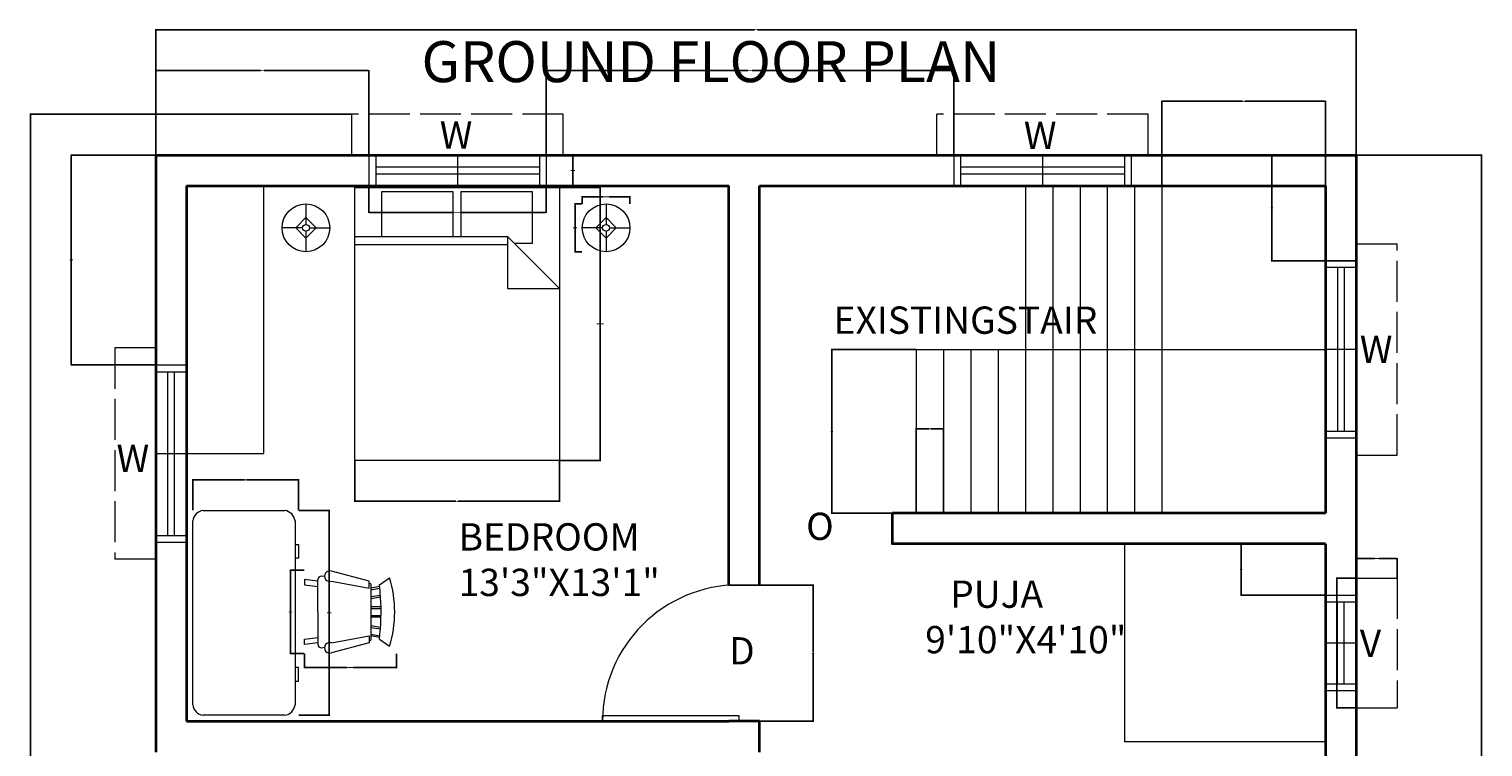
# Model space of a CAD drawing. Units: inches. Extents: x -35 to 832, y -515 to 219.
# Tile 5 of 7: x -35 to 391, y 9 to 219. Entities that reach past the tile are written whole.
import ezdxf

# ---------------------------------------------------------------- set-up
doc = ezdxf.new("R2010")
doc.units = ezdxf.units.IN
doc.header["$MEASUREMENT"] = 0
doc.linetypes.add('ACAD_ISO02W100', pattern=[15, 12, -3])
for name, color, linetype, lineweight in [('A-ANNO-TEXT', 7, 'Continuous', 18), ('A-AREA-IDEN', 7, 'Continuous', 18), ('A-DOOR', 4, 'Continuous', 18), ('A-FLOR-CASE', 3, 'Continuous', 18), ('A-FLOR-STRS', 2, 'Continuous', 18), ('A-FURN', 8, 'Continuous', 18), ('A-GLAZ', 2, 'Continuous', 18), ('A-GLAZ-OVHD', 2, 'ACAD_ISO02W100', 13), ('A-WALL', 10, 'Continuous', 35), ('G-ANNO-TEXT', 7, 'Continuous', 35), ('S-ANNO-DIMS', 2, 'Continuous', 18)]:
    doc.layers.add(name, color=color, linetype=linetype, lineweight=lineweight)
doc.styles.get("Standard").update_dxf_attribs({"font": 'arial.ttf'})
doc.dimstyles.get("Standard").update_dxf_attribs({"dimtxt": 0.18, "dimasz": 0.18, "dimexe": 0.18, "dimexo": 0.0625, "dimgap": 0.09, "dimtad": 0, "dimtih": 1, "dimtoh": 1, "dimdec": 1, "dimzin": 0, "dimdsep": 46, "dimlunit": 4, "dimtxsty": 'Standard', "dimcen": 0.09, "dimclrd": 211, "dimclre": 4, "dimclrt": 3, "dimadec": 0, "dimazin": 0, "dimtfac": 0.5, "dimtdec": 1, "dimtofl": 0, "dimtmove": 0, "dimatfit": 3, "dimfxl": 1, "dimtfill": 2, "dimtfillclr": 61, "dimtolj": 1, "dimtzin": 0, "dimarcsym": 0})

# ---------------------------------------------------------------- blocks, each defined once
blk = doc.blocks.new('*U5')
for p, q in [((0, 0), (0, -6)), ((40, 0), (40, -6))]:
    blk.add_line(p, q)
blk.add_lwpolyline([(0, 0), (0, 40), (1.75, 40), (1.75, 0)], close=True)
blk.add_arc((0, 0), 40, 0, 90)
blk = doc.blocks.new('Bed - Queen')
for p, q in [((0, -80.00003), (0, 0)), ((0, 0), (59.99999, 0)), ((59.99999, 0), (59.99999, -80.00003)), ((7.99999, -1.2), (28.79998, -1.2)), ((7.99999, -14.4), (7.99999, -1.2)), ((28.79998, -1.2), (28.79998, -14.4)), ((31.19999, -1.2), (51.99999, -1.2)), ((31.19999, -14.4), (31.19999, -1.2)), ((51.99999, -1.2), (51.99999, -16.4)), ((0, -14.4), (44.8, -14.4)), ((44.8, -16.8), (0, -16.8)), ((59.99999, -29.6), (44.8, -14.4)), ((44.8, -14.4), (44.8, -29.6)), ((51.99999, -16.4), (46.79936, -16.4)), ((44.8, -29.6), (59.99999, -29.6)), ((59.99999, -80.00003), (0, -80.00003))]:
    blk.add_line(p, q)
blk = doc.blocks.new('Chair - Rocking')
for p, q in [((-8, -4.5), (-10, -1.5)), ((-4.5, -7), (-4.96674, -4.19951)), ((-4, -7), (-4.40532, -4.16272)), ((-1.5, -4.05012), (-1.5, -7)), ((-1, -7), (-1, -4.05012)), ((1, -7), (1, -4.04655)), ((1.5, -4.05012), (1.5, -7)), ((4, -7), (4.40187, -4.18694)), ((4.5, -7), (4.96761, -4.19437)), ((8, -4.5), (10, -1.5)), ((-9, -7.5), (-12, -18.49999)), ((-7, -7.5), (-9, -7.5)), ((-9, -18.49999), (-7, -7.5)), ((-8.23428, -6.99939), (-8.3093, -7.47958)), ((-8.23041, -7), (8.23915, -7)), ((-7.5, -4.5), (-7, -7)), ((-6.5, -7), (-7.02225, -4.43)), ((6.5, -7), (7, -4.4057)), ((7.5, -4.5), (7, -7)), ((7, -7.5), (9, -7.5)), ((9, -18.49999), (7, -7.5)), ((8.31071, -7.48854), (8.23449, -7.00073)), ((9, -7.5), (12, -18.49999)), ((-10.36644, -20.64523), (-10.5, -21.49999)), ((10.5, -21.49999), (10.3575, -20.58798)), ((-9, -22.49999), (-9.5, -26.49999)), ((0, -22.49999), (-9.5, -22.49999)), ((-8, -26.49999), (-7.5, -22.49999)), ((0, -22.49999), (9.5, -22.49999)), ((8, -26.49999), (7.5, -22.49999)), ((9, -22.49999), (9.5, -26.49999)), ((-9.5, -26.49999), (-8, -26.49999)), ((9.5, -26.49999), (8, -26.49999))]:
    blk.add_line(p, q)
for centre, radius, start, end in [((0, -34.08333), 34.08333, 72.93847, 107.0615), ((0, -68.25004), 64.25, 93.92211, 97.15267), ((0, -68.25004), 64.25, 82.84733, 93.92211), ((-10.5, -18.99999), 1.58114, 161.5651, 18.43495), ((10.5, -18.99999), 1.58114, 161.5651, 18.43495), ((-9.5, -21.49999), 1, 180, 270), ((9.5, -21.49999), 1, 270, 0)]:
    blk.add_arc(centre, radius, start, end)
blk = doc.blocks.new('Desk - 30 x 60 in.')
for p, q in [((-26.999995, 0), (26.999995, 0)), ((-29.999995, -27), (-29.999995, -3)), ((29.999995, -3), (29.999995, -27)), ((26.999995, -30), (-26.999995, -30)), ((-20.000005, -30), (-20.000005, -31)), ((-20.000005, -31), (-16.000005, -31)), ((-16.000005, -31), (-16.000005, -30)), ((15.999995, -31), (15.999995, -30)), ((19.999995, -31), (15.999995, -31)), ((19.999995, -30), (19.999995, -31))]:
    blk.add_line(p, q)
for centre, start, end in [((-26.499995, -3.5), 98.1301, 171.8699), ((26.499995, -3.5), 8.130102, 81.8699), ((-26.499995, -26.5), 188.1301, 261.8699), ((26.499995, -26.5), 278.1301, 351.8699)]:
    blk.add_arc(centre, 3.535534, start, end)
blk = doc.blocks.new('Lamp - Table')
for p, q in [((0, 7), (0, 1)), ((-1, 0), (-7, 0)), ((0, 3), (-3, 0)), ((-3, 0), (0, -3)), ((3, 0), (0, 3)), ((0, -3), (3, 0)), ((1, 0), (7, 0)), ((0, -1), (0, -7))]:
    blk.add_line(p, q)
for radius in [7, 1]:
    blk.add_circle((0, 0), radius)
blk = doc.blocks.new('WIN-48')
for p, q in [((0, 9), (0, 0)), ((2, 9), (2, 0)), ((26, 9), (26, 0)), ((50, 9), (50, 0)), ((52, 9), (52, 0)), ((2, 5.5), (50, 5.5)), ((2, 3.5), (50, 3.5))]:
    blk.add_line(p, q)
blk = doc.blocks.new('VENT-24')
for p, q in [((9, 28), (0, 28)), ((9, 26), (0, 26)), ((3.5, 26), (3.5, 2)), ((5.5, 26), (5.5, 2)), ((9, 14), (0, 14)), ((9, 2), (0, 2)), ((9, 0), (0, 0))]:
    blk.add_line(p, q)
blk = doc.blocks.new('WIN-48-HOOD')
for p, q in [((5, 12), (0, 12)), ((0, 12), (0, 0)), ((57, 12), (62, 12)), ((62, 12), (62, 0)), ((0, 0), (62, 0))]:
    blk.add_line(p, q)
blk = doc.blocks.new('VENT-24-HOOD')
for p, q in [((12, 38), (0, 38)), ((0, 0), (0, 38)), ((12, 33), (12, 38)), ((12, 5), (12, 0)), ((12, 0), (0, 0))]:
    blk.add_line(p, q)
blk = doc.blocks.new('*D61')
at = {"layer": 'Defpoints', "color": 0, "transparency": 16777216}
for p in [(64.3, 173.05), (116.3, 173.05), (116.3, 165.25)]:
    blk.add_point(p, dxfattribs=at)
at = {"layer": 'S-ANNO-DIMS', "color": 4, "lineweight": -2, "transparency": 16777216}
for p, q in [((64.3, 172.99), (64.3, 165.07)), ((116.3, 172.99), (116.3, 165.07))]:
    blk.add_line(p, q, dxfattribs=at)
at = {"layer": 'S-ANNO-DIMS', "color": 211, "lineweight": -2, "transparency": 16777216}
for p, q in [((64.48, 165.25), (89.07, 165.25)), ((116.12, 165.25), (91.53, 165.25))]:
    blk.add_line(p, q, dxfattribs=at)
at = {"layer": 'S-ANNO-DIMS', "color": 211, "transparency": 16777216}
for points in [[(64.48, 165.28), (64.48, 165.22), (64.3, 165.25)], [(116.12, 165.28), (116.12, 165.22), (116.3, 165.25)]]:
    blk.add_solid(points, dxfattribs=at)
at = {"layer": 'S-ANNO-DIMS', "color": 3, "transparency": 16777216, "insert": (90.3, 165.25), "char_height": 0.18, "attachment_point": 5, "bg_fill": 1, "box_fill_scale": 1.25, "bg_fill_color": 61, "bg_fill_transparency": 0}
blk.add_mtext('\\A1;WINDOW 4\'-4" TYP.', dxfattribs=at)
blk = doc.blocks.new('*D62')
at = {"layer": 'Defpoints', "color": 0, "transparency": 16777216}
for p in [(116.3, 182.05), (124.1, 182.05), (116.3, 173.05)]:
    blk.add_point(p, dxfattribs=at)
at = {"layer": 'S-ANNO-DIMS', "color": 4, "lineweight": -2, "transparency": 16777216}
for p, q in [((116.36, 182.05), (124.28, 182.05)), ((116.36, 173.05), (124.28, 173.05))]:
    blk.add_line(p, q, dxfattribs=at)
at = {"layer": 'S-ANNO-DIMS', "color": 211, "lineweight": -2, "transparency": 16777216}
for p, q in [((124.1, 181.87), (124.1, 177.73)), ((124.1, 173.23), (124.1, 177.37))]:
    blk.add_line(p, q, dxfattribs=at)
at = {"layer": 'S-ANNO-DIMS', "color": 211, "transparency": 16777216}
for points in [[(124.07, 181.87), (124.13, 181.87), (124.1, 182.05)], [(124.07, 173.23), (124.13, 173.23), (124.1, 173.05)]]:
    blk.add_solid(points, dxfattribs=at)
at = {"layer": 'S-ANNO-DIMS', "color": 3, "transparency": 16777216, "insert": (124.1, 177.55), "char_height": 0.18, "attachment_point": 5, "bg_fill": 1, "box_fill_scale": 1.25, "bg_fill_color": 61, "bg_fill_transparency": 0}
blk.add_mtext('\\A1;0\'-9" TYP.', dxfattribs=at)
blk = doc.blocks.new('*D67')
at = {"layer": 'Defpoints', "color": 0, "transparency": 16777216}
for p in [(353.8, 58.05), (348.1, 20.05), (353.8, 20.05)]:
    blk.add_point(p, dxfattribs=at)
at = {"layer": 'S-ANNO-DIMS', "color": 4, "lineweight": -2, "transparency": 16777216}
for p, q in [((353.74, 58.05), (347.92, 58.05)), ((353.74, 20.05), (347.92, 20.05))]:
    blk.add_line(p, q, dxfattribs=at)
at = {"layer": 'S-ANNO-DIMS', "color": 211, "lineweight": -2, "transparency": 16777216}
for p, q in [((348.1, 57.87), (348.1, 39.23)), ((348.1, 20.23), (348.1, 38.87))]:
    blk.add_line(p, q, dxfattribs=at)
at = {"layer": 'S-ANNO-DIMS', "color": 211, "transparency": 16777216}
for points in [[(348.07, 57.87), (348.13, 57.87), (348.1, 58.05)], [(348.07, 20.23), (348.13, 20.23), (348.1, 20.05)]]:
    blk.add_solid(points, dxfattribs=at)
at = {"layer": 'S-ANNO-DIMS', "color": 3, "transparency": 16777216, "insert": (348.1, 39.05), "char_height": 0.18, "attachment_point": 5, "bg_fill": 1, "box_fill_scale": 1.25, "bg_fill_color": 61, "bg_fill_transparency": 0}
blk.add_mtext('\\A1;VENT HOOD 3\'-2" TYP.', dxfattribs=at)
blk = doc.blocks.new('*D68')
at = {"layer": 'Defpoints', "color": 0, "transparency": 16777216}
for p in [(353.8, 63.75), (353.8, 58.05), (365.8, 58.05)]:
    blk.add_point(p, dxfattribs=at)
at = {"layer": 'S-ANNO-DIMS', "color": 4, "lineweight": -2, "transparency": 16777216}
for p, q in [((353.8, 58.11), (353.8, 63.93)), ((365.8, 58.11), (365.8, 63.93))]:
    blk.add_line(p, q, dxfattribs=at)
at = {"layer": 'S-ANNO-DIMS', "color": 211, "lineweight": -2, "transparency": 16777216}
for p, q in [((353.98, 63.75), (359.17, 63.75)), ((365.62, 63.75), (360.43, 63.75))]:
    blk.add_line(p, q, dxfattribs=at)
at = {"layer": 'S-ANNO-DIMS', "color": 211, "transparency": 16777216}
for points in [[(353.98, 63.78), (353.98, 63.72), (353.8, 63.75)], [(365.62, 63.78), (365.62, 63.72), (365.8, 63.75)]]:
    blk.add_solid(points, dxfattribs=at)
at = {"layer": 'S-ANNO-DIMS', "color": 3, "transparency": 16777216, "insert": (359.8, 63.75), "char_height": 0.18, "attachment_point": 5, "bg_fill": 1, "box_fill_scale": 1.25, "bg_fill_color": 61, "bg_fill_transparency": 0}
blk.add_mtext('\\A1;1\'-0" TYP.', dxfattribs=at)
blk = doc.blocks.new('*D73')
at = {"layer": 'Defpoints', "color": 0, "transparency": 16777216}
for p in [(126.84, 167.72), (140.84, 169.82), (140.84, 167.72)]:
    blk.add_point(p, dxfattribs=at)
at = {"layer": 'S-ANNO-DIMS', "color": 4, "lineweight": -2, "transparency": 16777216}
for p, q in [((126.84, 167.79), (126.84, 170)), ((140.84, 167.79), (140.84, 170))]:
    blk.add_line(p, q, dxfattribs=at)
at = {"layer": 'S-ANNO-DIMS', "color": 211, "lineweight": -2, "transparency": 16777216}
for p, q in [((127.02, 169.82), (132.83, 169.82)), ((140.66, 169.82), (134.85, 169.82))]:
    blk.add_line(p, q, dxfattribs=at)
at = {"layer": 'S-ANNO-DIMS', "color": 211, "transparency": 16777216}
for points in [[(127.02, 169.85), (127.02, 169.79), (126.84, 169.82)], [(140.66, 169.85), (140.66, 169.79), (140.84, 169.82)]]:
    blk.add_solid(points, dxfattribs=at)
at = {"layer": 'S-ANNO-DIMS', "color": 3, "transparency": 16777216, "insert": (133.84, 169.82), "char_height": 0.18, "attachment_point": 5, "bg_fill": 1, "box_fill_scale": 1.25, "bg_fill_color": 61, "bg_fill_transparency": 0}
blk.add_mtext('\\A1;LAMP 1\'-2" TYP.', dxfattribs=at)
blk = doc.blocks.new('*D74')
at = {"layer": 'Defpoints', "color": 0, "transparency": 16777216}
for p in [(124.74, 167.72), (126.84, 167.72), (126.84, 153.72)]:
    blk.add_point(p, dxfattribs=at)
at = {"layer": 'S-ANNO-DIMS', "color": 4, "lineweight": -2, "transparency": 16777216}
for p, q in [((126.78, 167.72), (124.56, 167.72)), ((126.78, 153.72), (124.56, 153.72))]:
    blk.add_line(p, q, dxfattribs=at)
at = {"layer": 'S-ANNO-DIMS', "color": 211, "lineweight": -2, "transparency": 16777216}
for p, q in [((124.74, 167.54), (124.74, 160.9)), ((124.74, 153.9), (124.74, 160.54))]:
    blk.add_line(p, q, dxfattribs=at)
at = {"layer": 'S-ANNO-DIMS', "color": 211, "transparency": 16777216}
for points in [[(124.71, 167.54), (124.77, 167.54), (124.74, 167.72)], [(124.71, 153.9), (124.77, 153.9), (124.74, 153.72)]]:
    blk.add_solid(points, dxfattribs=at)
at = {"layer": 'S-ANNO-DIMS', "color": 3, "transparency": 16777216, "insert": (124.74, 160.72), "char_height": 0.18, "attachment_point": 5, "bg_fill": 1, "box_fill_scale": 1.25, "bg_fill_color": 61, "bg_fill_transparency": 0}
blk.add_mtext('\\A1;1\'-2" TYP.', dxfattribs=at)
blk = doc.blocks.new('*D89')
at = {"layer": 'Defpoints', "color": 0, "transparency": 16777216}
for p in [(120.14, 172.55), (132.14, 172.55), (120.14, 92.55)]:
    blk.add_point(p, dxfattribs=at)
at = {"layer": 'S-ANNO-DIMS', "color": 4, "lineweight": -2, "transparency": 16777216}
for p, q in [((120.2, 172.55), (132.32, 172.55)), ((120.2, 92.55), (132.32, 92.55))]:
    blk.add_line(p, q, dxfattribs=at)
at = {"layer": 'S-ANNO-DIMS', "color": 211, "lineweight": -2, "transparency": 16777216}
for p, q in [((132.14, 172.37), (132.14, 132.74)), ((132.14, 92.73), (132.14, 132.36))]:
    blk.add_line(p, q, dxfattribs=at)
at = {"layer": 'S-ANNO-DIMS', "color": 211, "transparency": 16777216}
for points in [[(132.11, 172.37), (132.17, 172.37), (132.14, 172.55)], [(132.11, 92.73), (132.17, 92.73), (132.14, 92.55)]]:
    blk.add_solid(points, dxfattribs=at)
at = {"layer": 'S-ANNO-DIMS', "color": 3, "transparency": 16777216, "insert": (132.14, 132.55), "char_height": 0.18, "attachment_point": 5, "bg_fill": 1, "box_fill_scale": 1.25, "bg_fill_color": 61, "bg_fill_transparency": 0}
blk.add_mtext('\\A1;QUEEN BED 6\'-8"', dxfattribs=at)
blk = doc.blocks.new('*D90')
at = {"layer": 'Defpoints', "color": 0, "transparency": 16777216}
for p in [(60.14, 92.55), (120.14, 92.55), (120.14, 80.55)]:
    blk.add_point(p, dxfattribs=at)
at = {"layer": 'S-ANNO-DIMS', "color": 4, "lineweight": -2, "transparency": 16777216}
for p, q in [((60.14, 92.49), (60.14, 80.37)), ((120.14, 92.49), (120.14, 80.37))]:
    blk.add_line(p, q, dxfattribs=at)
at = {"layer": 'S-ANNO-DIMS', "color": 211, "lineweight": -2, "transparency": 16777216}
for p, q in [((60.32, 80.55), (89.81, 80.55)), ((119.96, 80.55), (90.47, 80.55))]:
    blk.add_line(p, q, dxfattribs=at)
at = {"layer": 'S-ANNO-DIMS', "color": 211, "transparency": 16777216}
for points in [[(60.32, 80.58), (60.32, 80.52), (60.14, 80.55)], [(119.96, 80.58), (119.96, 80.52), (120.14, 80.55)]]:
    blk.add_solid(points, dxfattribs=at)
at = {"layer": 'S-ANNO-DIMS', "color": 3, "transparency": 16777216, "insert": (90.14, 80.55), "char_height": 0.18, "attachment_point": 5, "bg_fill": 1, "box_fill_scale": 1.25, "bg_fill_color": 61, "bg_fill_transparency": 0}
blk.add_mtext('\\A1;5\'-0"', dxfattribs=at)
blk = doc.blocks.new('*D91')
at = {"layer": 'Defpoints', "color": 0, "transparency": 16777216}
for p in [(45.37, 35.89), (72.37, 35.89), (72.37, 31.84)]:
    blk.add_point(p, dxfattribs=at)
at = {"layer": 'S-ANNO-DIMS', "color": 4, "lineweight": -2, "transparency": 16777216}
for p, q in [((45.37, 35.82), (45.37, 31.66)), ((72.37, 35.82), (72.37, 31.66))]:
    blk.add_line(p, q, dxfattribs=at)
at = {"layer": 'S-ANNO-DIMS', "color": 211, "lineweight": -2, "transparency": 16777216}
for p, q in [((45.55, 31.84), (57.97, 31.84)), ((72.19, 31.84), (59.77, 31.84))]:
    blk.add_line(p, q, dxfattribs=at)
at = {"layer": 'S-ANNO-DIMS', "color": 211, "transparency": 16777216}
for points in [[(45.55, 31.87), (45.55, 31.81), (45.37, 31.84)], [(72.19, 31.87), (72.19, 31.81), (72.37, 31.84)]]:
    blk.add_solid(points, dxfattribs=at)
at = {"layer": 'S-ANNO-DIMS', "color": 3, "transparency": 16777216, "insert": (58.87, 31.84), "char_height": 0.18, "attachment_point": 5, "bg_fill": 1, "box_fill_scale": 1.25, "bg_fill_color": 61, "bg_fill_transparency": 0}
blk.add_mtext('\\A1;ROCKER 2\'-3"', dxfattribs=at)
blk = doc.blocks.new('*D92')
at = {"layer": 'Defpoints', "color": 0, "transparency": 16777216}
for p in [(45.37, 60.32), (41.32, 35.89), (45.37, 35.89)]:
    blk.add_point(p, dxfattribs=at)
at = {"layer": 'S-ANNO-DIMS', "color": 4, "lineweight": -2, "transparency": 16777216}
for p, q in [((45.31, 60.32), (41.14, 60.32)), ((45.31, 35.89), (41.14, 35.89))]:
    blk.add_line(p, q, dxfattribs=at)
at = {"layer": 'S-ANNO-DIMS', "color": 211, "lineweight": -2, "transparency": 16777216}
for p, q in [((41.32, 60.14), (41.32, 48.29)), ((41.32, 36.07), (41.32, 47.92))]:
    blk.add_line(p, q, dxfattribs=at)
at = {"layer": 'S-ANNO-DIMS', "color": 211, "transparency": 16777216}
for points in [[(41.29, 60.14), (41.35, 60.14), (41.32, 60.32)], [(41.29, 36.07), (41.35, 36.07), (41.32, 35.89)]]:
    blk.add_solid(points, dxfattribs=at)
at = {"layer": 'S-ANNO-DIMS', "color": 3, "transparency": 16777216, "insert": (41.32, 48.1), "char_height": 0.18, "attachment_point": 5, "bg_fill": 1, "box_fill_scale": 1.25, "bg_fill_color": 61, "bg_fill_transparency": 0}
blk.add_mtext('\\A1;2\'-0 1/2"', dxfattribs=at)
blk = doc.blocks.new('*D93')
at = {"layer": 'Defpoints', "color": 0, "transparency": 16777216}
for p in [(43.66, 77.85), (52.66, 77.85), (43.66, 17.85)]:
    blk.add_point(p, dxfattribs=at)
at = {"layer": 'S-ANNO-DIMS', "color": 4, "lineweight": -2, "transparency": 16777216}
for p, q in [((43.72, 77.85), (52.84, 77.85)), ((43.72, 17.85), (52.84, 17.85))]:
    blk.add_line(p, q, dxfattribs=at)
at = {"layer": 'S-ANNO-DIMS', "color": 211, "lineweight": -2, "transparency": 16777216}
for p, q in [((52.66, 77.67), (52.66, 48.03)), ((52.66, 18.03), (52.66, 47.67))]:
    blk.add_line(p, q, dxfattribs=at)
at = {"layer": 'S-ANNO-DIMS', "color": 211, "transparency": 16777216}
for points in [[(52.63, 77.67), (52.69, 77.67), (52.66, 77.85)], [(52.63, 18.03), (52.69, 18.03), (52.66, 17.85)]]:
    blk.add_solid(points, dxfattribs=at)
at = {"layer": 'S-ANNO-DIMS', "color": 3, "transparency": 16777216, "insert": (52.66, 47.85), "char_height": 0.18, "attachment_point": 5, "bg_fill": 1, "box_fill_scale": 1.25, "bg_fill_color": 61, "bg_fill_transparency": 0}
blk.add_mtext('\\A1;DESK 5\'-0"', dxfattribs=at)
blk = doc.blocks.new('*D94')
at = {"layer": 'Defpoints', "color": 0, "transparency": 16777216}
for p in [(12.66, 86.85), (12.66, 77.85), (43.66, 77.85)]:
    blk.add_point(p, dxfattribs=at)
at = {"layer": 'S-ANNO-DIMS', "color": 4, "lineweight": -2, "transparency": 16777216}
for p, q in [((12.66, 77.91), (12.66, 87.03)), ((43.66, 77.91), (43.66, 87.03))]:
    blk.add_line(p, q, dxfattribs=at)
at = {"layer": 'S-ANNO-DIMS', "color": 211, "lineweight": -2, "transparency": 16777216}
for p, q in [((12.84, 86.85), (27.83, 86.85)), ((43.48, 86.85), (28.49, 86.85))]:
    blk.add_line(p, q, dxfattribs=at)
at = {"layer": 'S-ANNO-DIMS', "color": 211, "transparency": 16777216}
for points in [[(12.84, 86.88), (12.84, 86.82), (12.66, 86.85)], [(43.48, 86.88), (43.48, 86.82), (43.66, 86.85)]]:
    blk.add_solid(points, dxfattribs=at)
at = {"layer": 'S-ANNO-DIMS', "color": 3, "transparency": 16777216, "insert": (28.16, 86.85), "char_height": 0.18, "attachment_point": 5, "bg_fill": 1, "box_fill_scale": 1.25, "bg_fill_color": 61, "bg_fill_transparency": 0}
blk.add_mtext('\\A1;2\'-7"', dxfattribs=at)
blk = doc.blocks.new('*D103')
at = {"layer": 'Defpoints', "color": 0, "transparency": 16777216}
for p in [(64.3, 206.8), (1.8, 182.05), (64.3, 182.05)]:
    blk.add_point(p, dxfattribs=at)
at = {"layer": 'S-ANNO-DIMS', "color": 4, "lineweight": -2, "transparency": 16777216}
for p, q in [((1.8, 182.11), (1.8, 206.98)), ((64.3, 182.11), (64.3, 206.98))]:
    blk.add_line(p, q, dxfattribs=at)
at = {"layer": 'S-ANNO-DIMS', "color": 211, "lineweight": -2, "transparency": 16777216}
for p, q in [((1.98, 206.8), (32.51, 206.8)), ((64.12, 206.8), (33.59, 206.8))]:
    blk.add_line(p, q, dxfattribs=at)
at = {"layer": 'S-ANNO-DIMS', "color": 211, "transparency": 16777216}
for points in [[(1.98, 206.83), (1.98, 206.77), (1.8, 206.8)], [(64.12, 206.83), (64.12, 206.77), (64.3, 206.8)]]:
    blk.add_solid(points, dxfattribs=at)
at = {"layer": 'S-ANNO-DIMS', "color": 3, "transparency": 16777216, "insert": (33.05, 206.8), "char_height": 0.18, "attachment_point": 5, "bg_fill": 1, "box_fill_scale": 1.25, "bg_fill_color": 61, "bg_fill_transparency": 0}
blk.add_mtext('\\A1;5\'-2 1/2"', dxfattribs=at)
blk = doc.blocks.new('*D104')
at = {"layer": 'Defpoints', "color": 0, "transparency": 16777216}
for p in [(235.8, 206.8), (116.3, 182.05), (235.8, 182.05)]:
    blk.add_point(p, dxfattribs=at)
at = {"layer": 'S-ANNO-DIMS', "color": 4, "lineweight": -2, "transparency": 16777216}
for p, q in [((116.3, 182.11), (116.3, 206.98)), ((235.8, 182.11), (235.8, 206.98))]:
    blk.add_line(p, q, dxfattribs=at)
at = {"layer": 'S-ANNO-DIMS', "color": 211, "lineweight": -2, "transparency": 16777216}
for p, q in [((116.48, 206.8), (175.44, 206.8)), ((235.62, 206.8), (176.66, 206.8))]:
    blk.add_line(p, q, dxfattribs=at)
at = {"layer": 'S-ANNO-DIMS', "color": 211, "transparency": 16777216}
for points in [[(116.48, 206.83), (116.48, 206.77), (116.3, 206.8)], [(235.62, 206.83), (235.62, 206.77), (235.8, 206.8)]]:
    blk.add_solid(points, dxfattribs=at)
at = {"layer": 'S-ANNO-DIMS', "color": 3, "transparency": 16777216, "insert": (176.05, 206.8), "char_height": 0.18, "attachment_point": 5, "bg_fill": 1, "box_fill_scale": 1.25, "bg_fill_color": 61, "bg_fill_transparency": 0}
blk.add_mtext('\\A1;9\'-11 1/2"', dxfattribs=at)
blk = doc.blocks.new('*D105')
at = {"layer": 'Defpoints', "color": 0, "transparency": 16777216}
for p in [(353.8, 218.8), (1.8, 182.05), (353.8, 182.05)]:
    blk.add_point(p, dxfattribs=at)
at = {"layer": 'S-ANNO-DIMS', "color": 4, "lineweight": -2, "transparency": 16777216}
for p, q in [((1.8, 182.11), (1.8, 218.98)), ((353.8, 182.11), (353.8, 218.98))]:
    blk.add_line(p, q, dxfattribs=at)
at = {"layer": 'S-ANNO-DIMS', "color": 211, "lineweight": -2, "transparency": 16777216}
for p, q in [((1.98, 218.8), (177.4, 218.8)), ((353.62, 218.8), (178.2, 218.8))]:
    blk.add_line(p, q, dxfattribs=at)
at = {"layer": 'S-ANNO-DIMS', "color": 211, "transparency": 16777216}
for points in [[(1.98, 218.83), (1.98, 218.77), (1.8, 218.8)], [(353.62, 218.83), (353.62, 218.77), (353.8, 218.8)]]:
    blk.add_solid(points, dxfattribs=at)
at = {"layer": 'S-ANNO-DIMS', "color": 3, "transparency": 16777216, "insert": (177.8, 218.8), "char_height": 0.18, "attachment_point": 5, "bg_fill": 1, "box_fill_scale": 1.25, "bg_fill_color": 61, "bg_fill_transparency": 0}
blk.add_mtext('\\A1;29\'-4"', dxfattribs=at)
blk = doc.blocks.new('*D106')
at = {"layer": 'Defpoints', "color": 0, "transparency": 16777216}
for p in [(353.8, 182.05), (353.8, -254.95), (390.55, -254.95)]:
    blk.add_point(p, dxfattribs=at)
at = {"layer": 'S-ANNO-DIMS', "color": 4, "lineweight": -2, "transparency": 16777216}
for p, q in [((353.86, 182.05), (390.73, 182.05)), ((353.86, -254.95), (390.73, -254.95))]:
    blk.add_line(p, q, dxfattribs=at)
at = {"layer": 'S-ANNO-DIMS', "color": 211, "lineweight": -2, "transparency": 16777216}
for p, q in [((390.55, 181.87), (390.55, -36.27)), ((390.55, -254.77), (390.55, -36.63))]:
    blk.add_line(p, q, dxfattribs=at)
at = {"layer": 'S-ANNO-DIMS', "color": 211, "transparency": 16777216}
for points in [[(390.52, 181.87), (390.58, 181.87), (390.55, 182.05)], [(390.52, -254.77), (390.58, -254.77), (390.55, -254.95)]]:
    blk.add_solid(points, dxfattribs=at)
at = {"layer": 'S-ANNO-DIMS', "color": 3, "transparency": 16777216, "insert": (390.55, -36.45), "char_height": 0.18, "attachment_point": 5, "bg_fill": 1, "box_fill_scale": 1.25, "bg_fill_color": 61, "bg_fill_transparency": 0}
blk.add_mtext('\\A1;36\'-5"', dxfattribs=at)
blk = doc.blocks.new('*D110')
at = {"layer": 'Defpoints', "color": 0, "transparency": 16777216}
for p in [(59.3, 194.05), (-34.95, -254.95), (129.8, -254.95)]:
    blk.add_point(p, dxfattribs=at)
at = {"layer": 'S-ANNO-DIMS', "color": 4, "lineweight": -2, "transparency": 16777216}
for p, q in [((59.24, 194.05), (-35.13, 194.05)), ((129.74, -254.95), (-35.13, -254.95))]:
    blk.add_line(p, q, dxfattribs=at)
at = {"layer": 'S-ANNO-DIMS', "color": 211, "lineweight": -2, "transparency": 16777216}
for p, q in [((-34.95, 193.87), (-34.95, -30.27)), ((-34.95, -254.77), (-34.95, -30.63))]:
    blk.add_line(p, q, dxfattribs=at)
at = {"layer": 'S-ANNO-DIMS', "color": 211, "transparency": 16777216}
for points in [[(-34.98, 193.87), (-34.92, 193.87), (-34.95, 194.05)], [(-34.98, -254.77), (-34.92, -254.77), (-34.95, -254.95)]]:
    blk.add_solid(points, dxfattribs=at)
at = {"layer": 'S-ANNO-DIMS', "color": 3, "transparency": 16777216, "insert": (-34.95, -30.45), "char_height": 0.18, "attachment_point": 5, "bg_fill": 1, "box_fill_scale": 1.25, "bg_fill_color": 61, "bg_fill_transparency": 0}
blk.add_mtext('\\A1;37\'-5"', dxfattribs=at)
blk = doc.blocks.new('*D112')
at = {"layer": 'Defpoints', "color": 0, "transparency": 16777216}
for p in [(169.8, 55.94), (169.8, 16.05), (194.55, 16.05)]:
    blk.add_point(p, dxfattribs=at)
at = {"layer": 'S-ANNO-DIMS', "color": 4, "lineweight": -2, "transparency": 16777216}
for p, q in [((169.86, 55.94), (194.73, 55.94)), ((169.86, 16.05), (194.73, 16.05))]:
    blk.add_line(p, q, dxfattribs=at)
at = {"layer": 'S-ANNO-DIMS', "color": 211, "lineweight": -2, "transparency": 16777216}
for p, q in [((194.55, 55.76), (194.55, 36.18)), ((194.55, 16.23), (194.55, 35.81))]:
    blk.add_line(p, q, dxfattribs=at)
at = {"layer": 'S-ANNO-DIMS', "color": 211, "transparency": 16777216}
for points in [[(194.52, 55.76), (194.58, 55.76), (194.55, 55.94)], [(194.52, 16.23), (194.58, 16.23), (194.55, 16.05)]]:
    blk.add_solid(points, dxfattribs=at)
at = {"layer": 'S-ANNO-DIMS', "color": 3, "transparency": 16777216, "insert": (194.55, 35.99), "char_height": 0.18, "attachment_point": 5, "bg_fill": 1, "box_fill_scale": 1.25, "bg_fill_color": 61, "bg_fill_transparency": 0}
blk.add_mtext('\\A1;3\'-4"', dxfattribs=at)
blk = doc.blocks.new('*D115')
at = {"layer": 'Defpoints', "color": 0, "transparency": 16777216}
for p in [(-22.95, 182.05), (1.8, 182.05), (1.8, 120.55)]:
    blk.add_point(p, dxfattribs=at)
at = {"layer": 'S-ANNO-DIMS', "color": 4, "lineweight": -2, "transparency": 16777216}
for p, q in [((1.74, 182.05), (-23.13, 182.05)), ((1.74, 120.55), (-23.13, 120.55))]:
    blk.add_line(p, q, dxfattribs=at)
at = {"layer": 'S-ANNO-DIMS', "color": 211, "lineweight": -2, "transparency": 16777216}
for p, q in [((-22.95, 181.87), (-22.95, 151.48)), ((-22.95, 120.73), (-22.95, 151.12))]:
    blk.add_line(p, q, dxfattribs=at)
at = {"layer": 'S-ANNO-DIMS', "color": 211, "transparency": 16777216}
for points in [[(-22.98, 181.87), (-22.92, 181.87), (-22.95, 182.05)], [(-22.98, 120.73), (-22.92, 120.73), (-22.95, 120.55)]]:
    blk.add_solid(points, dxfattribs=at)
at = {"layer": 'S-ANNO-DIMS', "color": 3, "transparency": 16777216, "insert": (-22.95, 151.3), "char_height": 0.18, "attachment_point": 5, "bg_fill": 1, "box_fill_scale": 1.25, "bg_fill_color": 61, "bg_fill_transparency": 0}
blk.add_mtext('\\A1;5\'-1 1/2"', dxfattribs=at)
blk = doc.blocks.new('*D118')
at = {"layer": 'Defpoints', "color": 0, "transparency": 16777216}
for p in [(329.05, 182.05), (353.8, 182.05), (353.8, 151.05)]:
    blk.add_point(p, dxfattribs=at)
at = {"layer": 'S-ANNO-DIMS', "color": 4, "lineweight": -2, "transparency": 16777216}
for p, q in [((353.74, 182.05), (328.87, 182.05)), ((353.74, 151.05), (328.87, 151.05))]:
    blk.add_line(p, q, dxfattribs=at)
at = {"layer": 'S-ANNO-DIMS', "color": 211, "lineweight": -2, "transparency": 16777216}
for p, q in [((329.05, 181.87), (329.05, 166.73)), ((329.05, 151.23), (329.05, 166.37))]:
    blk.add_line(p, q, dxfattribs=at)
at = {"layer": 'S-ANNO-DIMS', "color": 211, "transparency": 16777216}
for points in [[(329.02, 181.87), (329.08, 181.87), (329.05, 182.05)], [(329.02, 151.23), (329.08, 151.23), (329.05, 151.05)]]:
    blk.add_solid(points, dxfattribs=at)
at = {"layer": 'S-ANNO-DIMS', "color": 3, "transparency": 16777216, "insert": (329.05, 166.55), "char_height": 0.18, "attachment_point": 5, "bg_fill": 1, "box_fill_scale": 1.25, "bg_fill_color": 61, "bg_fill_transparency": 0}
blk.add_mtext('\\A1;2\'-7"', dxfattribs=at)
blk = doc.blocks.new('*D119')
at = {"layer": 'Defpoints', "color": 0, "transparency": 16777216}
for p in [(320.05, 68.05), (344.8, 68.05), (344.8, 53.05)]:
    blk.add_point(p, dxfattribs=at)
at = {"layer": 'S-ANNO-DIMS', "color": 4, "lineweight": -2, "transparency": 16777216}
for p, q in [((344.74, 68.05), (319.87, 68.05)), ((344.74, 53.05), (319.87, 53.05))]:
    blk.add_line(p, q, dxfattribs=at)
at = {"layer": 'S-ANNO-DIMS', "color": 211, "lineweight": -2, "transparency": 16777216}
for p, q in [((320.05, 67.87), (320.05, 60.73)), ((320.05, 53.23), (320.05, 60.37))]:
    blk.add_line(p, q, dxfattribs=at)
at = {"layer": 'S-ANNO-DIMS', "color": 211, "transparency": 16777216}
for points in [[(320.02, 67.87), (320.08, 67.87), (320.05, 68.05)], [(320.02, 53.23), (320.08, 53.23), (320.05, 53.05)]]:
    blk.add_solid(points, dxfattribs=at)
at = {"layer": 'S-ANNO-DIMS', "color": 3, "transparency": 16777216, "insert": (320.05, 60.55), "char_height": 0.18, "attachment_point": 5, "bg_fill": 1, "box_fill_scale": 1.25, "bg_fill_color": 61, "bg_fill_transparency": 0}
blk.add_mtext('\\A1;1\'-3"', dxfattribs=at)
blk = doc.blocks.new('*D122')
at = {"layer": 'Defpoints', "color": 0, "transparency": 16777216}
for p in [(200.05, 125.05), (224.8, 125.05), (224.8, 77.05)]:
    blk.add_point(p, dxfattribs=at)
at = {"layer": 'S-ANNO-DIMS', "color": 4, "lineweight": -2, "transparency": 16777216}
for p, q in [((224.74, 125.05), (199.87, 125.05)), ((224.74, 77.05), (199.87, 77.05))]:
    blk.add_line(p, q, dxfattribs=at)
at = {"layer": 'S-ANNO-DIMS', "color": 211, "lineweight": -2, "transparency": 16777216}
for p, q in [((200.05, 124.87), (200.05, 101.23)), ((200.05, 77.23), (200.05, 100.87))]:
    blk.add_line(p, q, dxfattribs=at)
at = {"layer": 'S-ANNO-DIMS', "color": 211, "transparency": 16777216}
for points in [[(200.02, 124.87), (200.08, 124.87), (200.05, 125.05)], [(200.02, 77.23), (200.08, 77.23), (200.05, 77.05)]]:
    blk.add_solid(points, dxfattribs=at)
at = {"layer": 'S-ANNO-DIMS', "color": 3, "transparency": 16777216, "insert": (200.05, 101.05), "char_height": 0.18, "attachment_point": 5, "bg_fill": 1, "box_fill_scale": 1.25, "bg_fill_color": 61, "bg_fill_transparency": 0}
blk.add_mtext('\\A1;4\'-0"', dxfattribs=at)
blk = doc.blocks.new('*D123')
at = {"layer": 'Defpoints', "color": 0, "transparency": 16777216}
for p in [(232.8, 101.8), (224.8, 77.05), (232.8, 77.05)]:
    blk.add_point(p, dxfattribs=at)
at = {"layer": 'S-ANNO-DIMS', "color": 4, "lineweight": -2, "transparency": 16777216}
for p, q in [((224.8, 77.11), (224.8, 101.98)), ((232.8, 77.11), (232.8, 101.98))]:
    blk.add_line(p, q, dxfattribs=at)
at = {"layer": 'S-ANNO-DIMS', "color": 211, "lineweight": -2, "transparency": 16777216}
for p, q in [((224.98, 101.8), (228.47, 101.8)), ((232.62, 101.8), (229.13, 101.8))]:
    blk.add_line(p, q, dxfattribs=at)
at = {"layer": 'S-ANNO-DIMS', "color": 211, "transparency": 16777216}
for points in [[(224.98, 101.83), (224.98, 101.77), (224.8, 101.8)], [(232.62, 101.83), (232.62, 101.77), (232.8, 101.8)]]:
    blk.add_solid(points, dxfattribs=at)
at = {"layer": 'S-ANNO-DIMS', "color": 3, "transparency": 16777216, "insert": (228.8, 101.8), "char_height": 0.18, "attachment_point": 5, "bg_fill": 1, "box_fill_scale": 1.25, "bg_fill_color": 61, "bg_fill_transparency": 0}
blk.add_mtext('\\A1;0\'-8"', dxfattribs=at)
blk = doc.blocks.new('*D124')
at = {"layer": 'Defpoints', "color": 0, "transparency": 16777216}
for p in [(344.8, 197.8), (296.8, 173.05), (344.8, 173.05)]:
    blk.add_point(p, dxfattribs=at)
at = {"layer": 'S-ANNO-DIMS', "color": 4, "lineweight": -2, "transparency": 16777216}
for p, q in [((296.8, 173.11), (296.8, 197.98)), ((344.8, 173.11), (344.8, 197.98))]:
    blk.add_line(p, q, dxfattribs=at)
at = {"layer": 'S-ANNO-DIMS', "color": 211, "lineweight": -2, "transparency": 16777216}
for p, q in [((296.98, 197.8), (320.47, 197.8)), ((344.62, 197.8), (321.13, 197.8))]:
    blk.add_line(p, q, dxfattribs=at)
at = {"layer": 'S-ANNO-DIMS', "color": 211, "transparency": 16777216}
for points in [[(296.98, 197.83), (296.98, 197.77), (296.8, 197.8)], [(344.62, 197.83), (344.62, 197.77), (344.8, 197.8)]]:
    blk.add_solid(points, dxfattribs=at)
at = {"layer": 'S-ANNO-DIMS', "color": 3, "transparency": 16777216, "insert": (320.8, 197.8), "char_height": 0.18, "attachment_point": 5, "bg_fill": 1, "box_fill_scale": 1.25, "bg_fill_color": 61, "bg_fill_transparency": 0}
blk.add_mtext('\\A1;4\'-0"', dxfattribs=at)

msp = doc.modelspace()

# ---------------------------------------------------------------- linework, layer by layer
at = {"layer": 'A-FLOR-CASE'}
for p, q in [((33.51, 94.55), (33.51, 173.05)), ((10.8, 94.55), (33.51, 94.55)), ((344.8, 10.05), (285.8, 10.05))]:
    msp.add_line(p, q, dxfattribs=at)
msp.add_lwpolyline([(285.8, 68.05), (285.8, 10.05)], dxfattribs=at)
at = {"layer": 'A-FLOR-STRS'}
for p, q in [((256.8, 173.05), (256.8, 77.05)), ((264.8, 173.05), (264.8, 77.05)), ((272.8, 173.05), (272.8, 77.05)), ((280.8, 173.05), (280.8, 77.05)), ((288.8, 173.05), (288.8, 77.05)), ((296.8, 173.05), (296.8, 77.05)), ((224.8, 125.05), (296.8, 125.05)), ((224.8, 125.05), (224.8, 77.05)), ((232.8, 125.05), (232.8, 77.05)), ((240.8, 125.05), (240.8, 77.05)), ((248.8, 125.05), (248.8, 77.05)), ((256.8, 125.05), (256.8, 77.05)), ((296.8, 125.05), (344.8, 125.05))]:
    msp.add_line(p, q, dxfattribs=at)
at = {"layer": 'A-WALL'}
for p, q in [((1.8, 182.05), (1.8, 7.05)), ((1.8, 182.05), (178.8, 182.05)), ((178.8, 182.05), (353.8, 182.05)), ((353.8, 182.05), (353.8, 77.05)), ((10.8, 173.05), (169.8, 173.05)), ((10.8, 173.05), (10.8, 16.05)), ((169.8, 55.94), (169.8, 173.05)), ((178.8, 173.05), (344.8, 173.05)), ((178.8, 55.94), (178.8, 173.05)), ((344.8, 173.05), (344.8, 77.05)), ((344.8, 77.05), (217.8, 77.05)), ((217.8, 67.85), (217.8, 77.05)), ((353.8, 77.05), (353.8, 10.05)), ((344.8, 68.05), (217.8, 68.05)), ((344.8, 68.05), (344.8, 10.05)), ((10.8, 16.05), (169.8, 16.05)), ((178.8, 16.05), (169.8, 16.05)), ((178.8, 7.05), (178.8, 16.05)), ((344.8, 10.05), (344.8, -140.95)), ((353.8, 10.05), (353.8, -140.95))]:
    msp.add_line(p, q, dxfattribs=at)

# ---------------------------------------------------------------- block references
at = {"layer": 'A-DOOR', "rotation": 90}
msp.add_blockref('*U5', (172.8, 16.05), dxfattribs=at)
at = {"layer": 'A-FURN'}
for name, p in [('Bed - Queen', (60.14, 172.55)), ('Lamp - Table', (45.84, 160.72)), ('Lamp - Table', (133.84, 160.72))]:
    msp.add_blockref(name, p, dxfattribs=at)
for name, p, rotation in [('Desk - 30 x 60 in.', (12.66, 47.85), 90), ('Chair - Rocking', (71.87, 48.1), 270)]:
    msp.add_blockref(name, p, dxfattribs=dict(at, rotation=rotation))
at = {"layer": 'A-GLAZ'}
for p in [(64.3, 173.05), (235.8, 173.05)]:
    msp.add_blockref('WIN-48', p, dxfattribs=at)
for name, p, rotation in [('WIN-48', (344.8, 151.05), 270.0000000000001), ('WIN-48', (10.8, 68.55), 90.00000000000003), ('VENT-24', (353.8, 53.05), 180)]:
    msp.add_blockref(name, p, dxfattribs=dict(at, rotation=rotation))
at = {"layer": 'A-GLAZ-OVHD'}
for name, p, rotation in [('WIN-48-HOOD', (121.3, 194.05), 180), ('WIN-48-HOOD', (292.8, 194.05), 180), ('WIN-48-HOOD', (365.8, 94.05), 89.9999999999998), ('WIN-48-HOOD', (-10.2, 125.55), 270), ('VENT-24-HOOD', (365.8, 58.05), 180)]:
    msp.add_blockref(name, p, dxfattribs=dict(at, rotation=rotation))

# ---------------------------------------------------------------- texts
at = {"layer": 'A-ANNO-TEXT'}
for s, p in [('W', (85.07, 183.95)), ('W', (256.33, 183.84)), ('W', (354.83, 121.14)), ('W', (-9.69, 89.14)), ('O', (192.5, 69.22)), ('V', (354.83, 34.95)), ('D', (169.91, 32.73))]:
    msp.add_text(s, height=8, dxfattribs=at).set_placement(p)
at = {"layer": 'A-AREA-IDEN', "char_height": 8, "attachment_point": 1}
for s, insert in [('EXISTINGSTAIR', (200.56, 137.65)), ('BEDROOM\\P13\'3"X13\'1"', (90.6, 74.12)), ('   PUJA\\P9\'10"X4\'10"', (227.41, 57.33))]:
    msp.add_mtext_dynamic_manual_height_columns(s, width=50.3004, gutter_width=1, heights=[0], dxfattribs=dict(at, insert=insert))
at = {"layer": 'G-ANNO-TEXT', "insert": (79.73, 215.43), "char_height": 12, "attachment_point": 1}
msp.add_mtext_dynamic_manual_height_columns('GROUND FLOOR PLAN', width=219.0757, gutter_width=1, heights=[0], dxfattribs=at)

# ---------------------------------------------------------------- dimensions: what is measured, and where the dimension line sits
at = {"layer": 'S-ANNO-DIMS'}
for base, p1, p2, picture, middle in [((353.8, 218.8), (1.8, 182.05), (353.8, 182.05), '*D105', (177.8, 218.8)), ((235.8, 206.8), (116.3, 182.05), (235.8, 182.05), '*D104', (176.05, 206.8)), ((344.8, 197.8), (296.8, 173.05), (344.8, 173.05), '*D124', (320.8, 197.8)), ((232.8, 101.8), (224.8, 77.05), (232.8, 77.05), '*D123', (228.8, 101.8)), ((120.14, 80.55), (60.14, 92.55), (120.14, 92.55), '*D90', (90.14, 80.55))]:
    dim = msp.add_linear_dim(base=base, p1=p1, p2=p2, dimstyle='Standard', override={"dimdec": 1, "dimlfac": 1, "dimrnd": 0, "dimzin": 1, "dimdsep": 46, "dimlunit": 4, "dimfrac": 2}, dxfattribs=at)
    dim.commit()
    dim.dimension.update_dxf_attribs({"geometry": picture, "text_midpoint": middle})
for base, p1, p2, angle, picture, middle in [((64.3, 206.8), (1.8, 182.05), (64.3, 182.05), 0, '*D103', (33.05, 206.8)), ((-34.95, -254.95), (59.3, 194.05), (129.8, -254.95), 90, '*D110', (-34.95, -30.45)), ((-22.95, 182.05), (1.8, 120.55), (1.8, 182.05), 90, '*D115', (-22.95, 151.3)), ((329.05, 182.05), (353.8, 151.05), (353.8, 182.05), 90, '*D118', (329.05, 166.55)), ((390.55, -254.95), (353.8, 182.05), (353.8, -254.95), 90, '*D106', (390.55, -36.45)), ((200.05, 125.05), (224.8, 77.05), (224.8, 125.05), 90, '*D122', (200.05, 101.05)), ((12.66, 86.85), (43.66, 77.85), (12.66, 77.85), 180, '*D94', (28.16, 86.85)), ((320.05, 68.05), (344.8, 53.05), (344.8, 68.05), 90, '*D119', (320.05, 60.55)), ((41.32, 35.89), (45.37, 60.32), (45.37, 35.89), 270, '*D92', (41.32, 48.1)), ((194.55, 16.05), (169.8, 55.94), (169.8, 16.05), 270, '*D112', (194.55, 35.99))]:
    dim = msp.add_linear_dim(base=base, p1=p1, p2=p2, angle=angle, dimstyle='Standard', override={"dimdec": 1, "dimlfac": 1, "dimrnd": 0, "dimzin": 1, "dimdsep": 46, "dimlunit": 4, "dimfrac": 2}, dxfattribs=at)
    dim.commit()
    dim.dimension.update_dxf_attribs({"geometry": picture, "text_midpoint": middle})
for base, p1, p2, angle, text, picture, middle in [((124.1, 182.05), (116.3, 173.05), (116.3, 182.05), 90, '<> TYP.', '*D62', (124.1, 177.55)), ((132.14, 172.55), (120.14, 92.55), (120.14, 172.55), 90, 'QUEEN BED <>', '*D89', (132.14, 132.55)), ((124.74, 167.72), (126.84, 153.72), (126.84, 167.72), 90, '<> TYP.', '*D74', (124.74, 160.72)), ((52.66, 77.85), (43.66, 17.85), (43.66, 77.85), 90, 'DESK <>', '*D93', (52.66, 47.85)), ((353.8, 63.75), (365.8, 58.05), (353.8, 58.05), 180, '<> TYP.', '*D68', (359.8, 63.75)), ((348.1, 20.05), (353.8, 58.05), (353.8, 20.05), 270, 'VENT HOOD <> TYP.', '*D67', (348.1, 39.05))]:
    dim = msp.add_linear_dim(base=base, p1=p1, p2=p2, angle=angle, text=text, dimstyle='Standard', override={"dimdec": 1, "dimlfac": 1, "dimrnd": 0, "dimzin": 1, "dimdsep": 46, "dimlunit": 4, "dimfrac": 2}, dxfattribs=at)
    dim.commit()
    dim.dimension.update_dxf_attribs({"geometry": picture, "text_midpoint": middle})
for base, p1, p2, text, picture, middle in [((116.3, 165.25), (64.3, 173.05), (116.3, 173.05), 'WINDOW <> TYP.', '*D61', (90.3, 165.25)), ((140.84, 169.82), (126.84, 167.72), (140.84, 167.72), 'LAMP <> TYP.', '*D73', (133.84, 169.82)), ((72.37, 31.84), (45.37, 35.89), (72.37, 35.89), 'ROCKER <>', '*D91', (58.87, 31.84))]:
    dim = msp.add_linear_dim(base=base, p1=p1, p2=p2, text=text, dimstyle='Standard', override={"dimdec": 1, "dimlfac": 1, "dimrnd": 0, "dimzin": 1, "dimdsep": 46, "dimlunit": 4, "dimfrac": 2}, dxfattribs=at)
    dim.commit()
    dim.dimension.update_dxf_attribs({"geometry": picture, "text_midpoint": middle})

doc.saveas('drawing.dxf')
